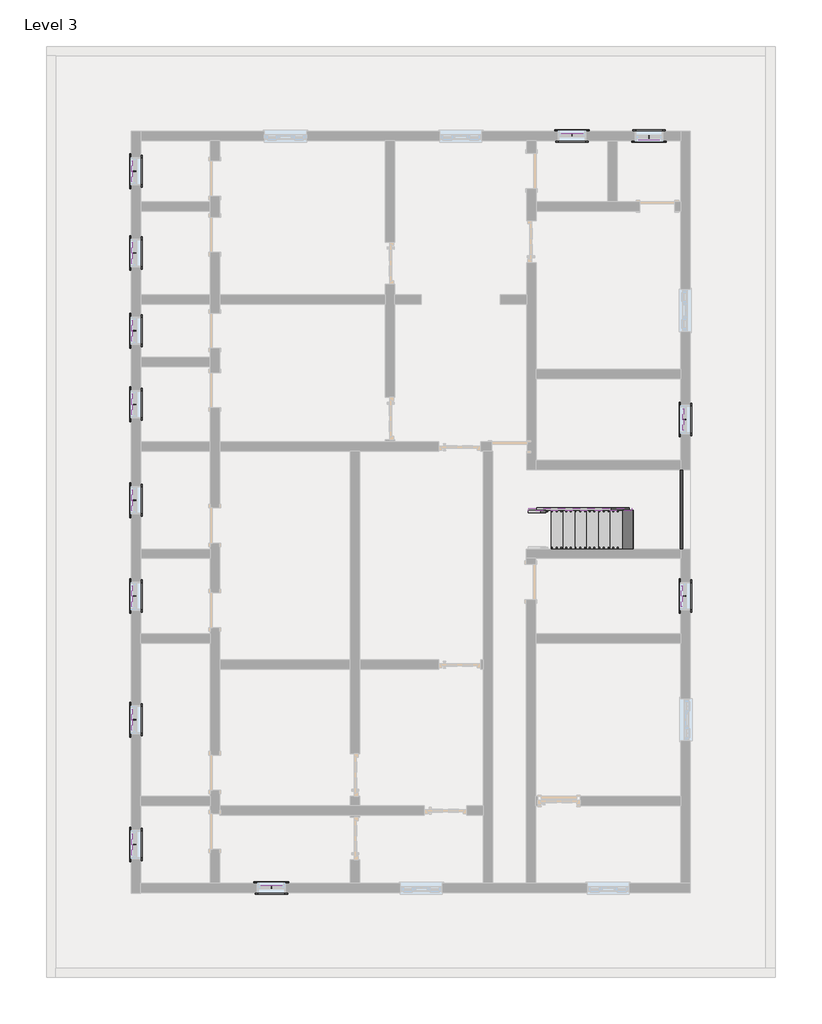
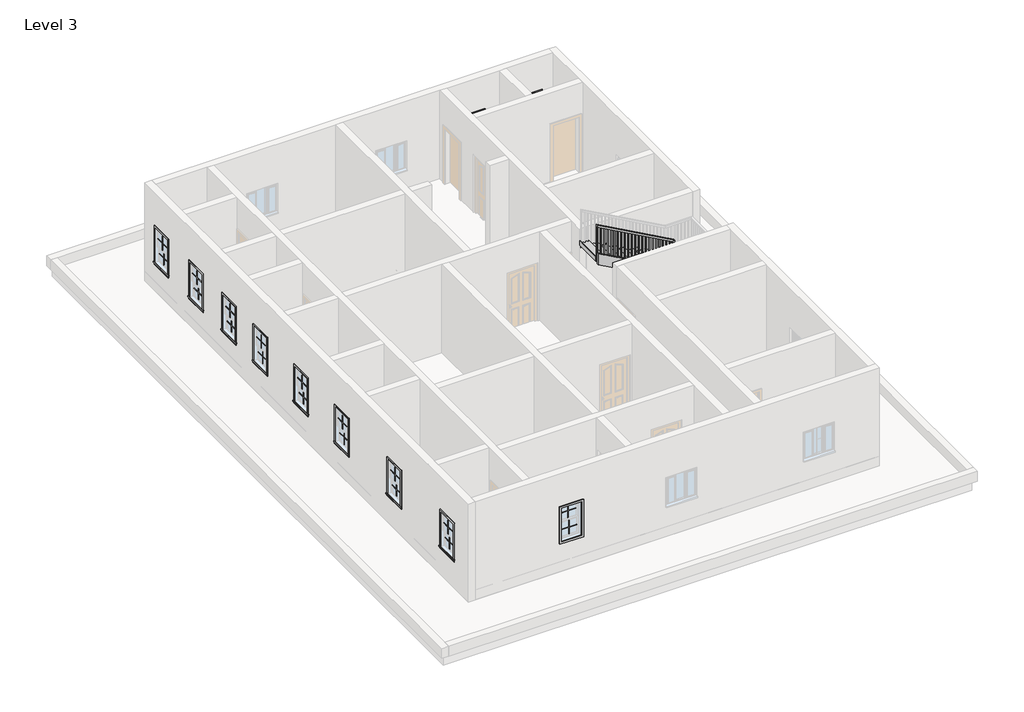
# One storey, part 3 of 3: 52 proxies, 5 members, 1 railing, 1 stair flight.
"""IFC4 building model written with IfcOpenShell, lengths in millimetres."""

from ifc_helpers import new_model, si_unit, frame, origin, place, context, project, spatial, polyline, outline, extrude, faceted_brep, transform, mapped, element, save
from components import muntin_pattern_2x2_muntin_pattern_2x2_eba6c5fb, trim_window_exterior_flat_with_sill_278e6a94, trim_window_interior_flat_picture_frame_e9fd5f45, stair_flight_fbd0abf4

model = new_model("IFC4")

# Units and contexts
model_context = context("Model", 3, world=origin())
ifc_project = project(units=[si_unit("LENGTHUNIT", "METRE", prefix="MILLI")], contexts=[model_context])

# Site, building, storey
site = spatial("IfcSite", under=ifc_project)
building = spatial("IfcBuilding", under=site)
storey = spatial("IfcBuildingStorey", under=building, Name="Level 3", Elevation=6096.0)

# Proxies
placement = place(None, origin())
muntin_pattern_2x2_muntin_pattern_2x2_shape = muntin_pattern_2x2_muntin_pattern_2x2_eba6c5fb(model_context)
element("IfcBuildingElementProxy", 1, Name="Muntin Pattern_2x2 : Muntin Pattern_2x2", ObjectType="Muntin Pattern_2x2 : Muntin Pattern_2x2", at=placement, inside=storey, context=model_context, shape_type="MappedRepresentation", body=[
    mapped(muntin_pattern_2x2_muntin_pattern_2x2_shape, transform((-10440.7626145, 6547.3404944, 7566.025), x_axis=(0.0, 1.0, 0.0), y_axis=(-1.0, 0.0, 0.0), z_axis=(0.0, 0.0, 1.0))),
])
element("IfcBuildingElementProxy", 2, Name="Muntin Pattern_2x2 : Muntin Pattern_2x2", ObjectType="Muntin Pattern_2x2 : Muntin Pattern_2x2", at=placement, inside=storey, context=model_context, shape_type="MappedRepresentation", body=[
    mapped(muntin_pattern_2x2_muntin_pattern_2x2_shape, transform((-10396.3126145, 6547.3404944, 7086.6), x_axis=(0.0, 1.0, 0.0), y_axis=(-1.0, 0.0, 0.0), z_axis=(0.0, 0.0, 1.0))),
])
element("IfcBuildingElementProxy", 3, Name="Muntin Pattern_2x2 : Muntin Pattern_2x2", ObjectType="Muntin Pattern_2x2 : Muntin Pattern_2x2", at=placement, inside=storey, context=model_context, shape_type="MappedRepresentation", body=[
    mapped(muntin_pattern_2x2_muntin_pattern_2x2_shape, transform((-10440.7626145, 4782.0404944, 7566.025), x_axis=(0.0, 1.0, 0.0), y_axis=(-1.0, 0.0, 0.0), z_axis=(0.0, 0.0, 1.0))),
])
element("IfcBuildingElementProxy", 4, Name="Muntin Pattern_2x2 : Muntin Pattern_2x2", ObjectType="Muntin Pattern_2x2 : Muntin Pattern_2x2", at=placement, inside=storey, context=model_context, shape_type="MappedRepresentation", body=[
    mapped(muntin_pattern_2x2_muntin_pattern_2x2_shape, transform((-10396.3126145, 4782.0404944, 7086.6), x_axis=(0.0, 1.0, 0.0), y_axis=(-1.0, 0.0, 0.0), z_axis=(0.0, 0.0, 1.0))),
])
element("IfcBuildingElementProxy", 5, Name="Muntin Pattern_2x2 : Muntin Pattern_2x2", ObjectType="Muntin Pattern_2x2 : Muntin Pattern_2x2", at=placement, inside=storey, context=model_context, shape_type="MappedRepresentation", body=[
    mapped(muntin_pattern_2x2_muntin_pattern_2x2_shape, transform((-10440.7626145, 3105.6404944, 7566.025), x_axis=(0.0, 1.0, 0.0), y_axis=(-1.0, 0.0, 0.0), z_axis=(0.0, 0.0, 1.0))),
])
element("IfcBuildingElementProxy", 6, Name="Muntin Pattern_2x2 : Muntin Pattern_2x2", ObjectType="Muntin Pattern_2x2 : Muntin Pattern_2x2", at=placement, inside=storey, context=model_context, shape_type="MappedRepresentation", body=[
    mapped(muntin_pattern_2x2_muntin_pattern_2x2_shape, transform((-10396.3126145, 3105.6404944, 7086.6), x_axis=(0.0, 1.0, 0.0), y_axis=(-1.0, 0.0, 0.0), z_axis=(0.0, 0.0, 1.0))),
])
element("IfcBuildingElementProxy", 7, Name="Muntin Pattern_2x2 : Muntin Pattern_2x2", ObjectType="Muntin Pattern_2x2 : Muntin Pattern_2x2", at=placement, inside=storey, context=model_context, shape_type="MappedRepresentation", body=[
    mapped(muntin_pattern_2x2_muntin_pattern_2x2_shape, transform((-10440.7626145, 1518.1404944, 7566.025), x_axis=(0.0, 1.0, 0.0), y_axis=(-1.0, 0.0, 0.0), z_axis=(0.0, 0.0, 1.0))),
])
element("IfcBuildingElementProxy", 8, Name="Muntin Pattern_2x2 : Muntin Pattern_2x2", ObjectType="Muntin Pattern_2x2 : Muntin Pattern_2x2", at=placement, inside=storey, context=model_context, shape_type="MappedRepresentation", body=[
    mapped(muntin_pattern_2x2_muntin_pattern_2x2_shape, transform((-10396.3126145, 1518.1404944, 7086.6), x_axis=(0.0, 1.0, 0.0), y_axis=(-1.0, 0.0, 0.0), z_axis=(0.0, 0.0, 1.0))),
])
element("IfcBuildingElementProxy", 9, Name="Muntin Pattern_2x2 : Muntin Pattern_2x2", ObjectType="Muntin Pattern_2x2 : Muntin Pattern_2x2", at=placement, inside=storey, context=model_context, shape_type="MappedRepresentation", body=[
    mapped(muntin_pattern_2x2_muntin_pattern_2x2_shape, transform((-10440.7626145, -551.9595056, 7566.025), x_axis=(0.0, 1.0, 0.0), y_axis=(-1.0, 0.0, 0.0), z_axis=(0.0, 0.0, 1.0))),
])
element("IfcBuildingElementProxy", 10, Name="Muntin Pattern_2x2 : Muntin Pattern_2x2", ObjectType="Muntin Pattern_2x2 : Muntin Pattern_2x2", at=placement, inside=storey, context=model_context, shape_type="MappedRepresentation", body=[
    mapped(muntin_pattern_2x2_muntin_pattern_2x2_shape, transform((-10396.3126145, -551.9595056, 7086.6), x_axis=(0.0, 1.0, 0.0), y_axis=(-1.0, 0.0, 0.0), z_axis=(0.0, 0.0, 1.0))),
])
element("IfcBuildingElementProxy", 11, Name="Muntin Pattern_2x2 : Muntin Pattern_2x2", ObjectType="Muntin Pattern_2x2 : Muntin Pattern_2x2", at=placement, inside=storey, context=model_context, shape_type="MappedRepresentation", body=[
    mapped(muntin_pattern_2x2_muntin_pattern_2x2_shape, transform((-10440.7626145, -2622.0595056, 7566.025), x_axis=(0.0, 1.0, 0.0), y_axis=(-1.0, 0.0, 0.0), z_axis=(0.0, 0.0, 1.0))),
])
element("IfcBuildingElementProxy", 12, Name="Muntin Pattern_2x2 : Muntin Pattern_2x2", ObjectType="Muntin Pattern_2x2 : Muntin Pattern_2x2", at=placement, inside=storey, context=model_context, shape_type="MappedRepresentation", body=[
    mapped(muntin_pattern_2x2_muntin_pattern_2x2_shape, transform((-10396.3126145, -2622.0595056, 7086.6), x_axis=(0.0, 1.0, 0.0), y_axis=(-1.0, 0.0, 0.0), z_axis=(0.0, 0.0, 1.0))),
])
element("IfcBuildingElementProxy", 13, Name="Muntin Pattern_2x2 : Muntin Pattern_2x2", ObjectType="Muntin Pattern_2x2 : Muntin Pattern_2x2", at=placement, inside=storey, context=model_context, shape_type="MappedRepresentation", body=[
    mapped(muntin_pattern_2x2_muntin_pattern_2x2_shape, transform((-10440.7626145, -5289.0595056, 7566.025), x_axis=(0.0, 1.0, 0.0), y_axis=(-1.0, 0.0, 0.0), z_axis=(0.0, 0.0, 1.0))),
])
element("IfcBuildingElementProxy", 14, Name="Muntin Pattern_2x2 : Muntin Pattern_2x2", ObjectType="Muntin Pattern_2x2 : Muntin Pattern_2x2", at=placement, inside=storey, context=model_context, shape_type="MappedRepresentation", body=[
    mapped(muntin_pattern_2x2_muntin_pattern_2x2_shape, transform((-10396.3126145, -5289.0595056, 7086.6), x_axis=(0.0, 1.0, 0.0), y_axis=(-1.0, 0.0, 0.0), z_axis=(0.0, 0.0, 1.0))),
])
element("IfcBuildingElementProxy", 15, Name="Muntin Pattern_2x2 : Muntin Pattern_2x2", ObjectType="Muntin Pattern_2x2 : Muntin Pattern_2x2", at=placement, inside=storey, context=model_context, shape_type="MappedRepresentation", body=[
    mapped(muntin_pattern_2x2_muntin_pattern_2x2_shape, transform((-10440.7626145, -7981.4595056, 7566.025), x_axis=(0.0, 1.0, 0.0), y_axis=(-1.0, 0.0, 0.0), z_axis=(0.0, 0.0, 1.0))),
])
element("IfcBuildingElementProxy", 16, Name="Muntin Pattern_2x2 : Muntin Pattern_2x2", ObjectType="Muntin Pattern_2x2 : Muntin Pattern_2x2", at=placement, inside=storey, context=model_context, shape_type="MappedRepresentation", body=[
    mapped(muntin_pattern_2x2_muntin_pattern_2x2_shape, transform((-10396.3126145, -7981.4595056, 7086.6), x_axis=(0.0, 1.0, 0.0), y_axis=(-1.0, 0.0, 0.0), z_axis=(0.0, 0.0, 1.0))),
])
element("IfcBuildingElementProxy", 17, Name="Muntin Pattern_2x2 : Muntin Pattern_2x2", ObjectType="Muntin Pattern_2x2 : Muntin Pattern_2x2", at=placement, inside=storey, context=model_context, shape_type="MappedRepresentation", body=[
    mapped(muntin_pattern_2x2_muntin_pattern_2x2_shape, transform((-7453.0876145, -8854.5845056, 7566.025), x_axis=(1.0, 0.0, 0.0), y_axis=(0.0, 1.0, 0.0), z_axis=(0.0, 0.0, 1.0))),
])
element("IfcBuildingElementProxy", 18, Name="Muntin Pattern_2x2 : Muntin Pattern_2x2", ObjectType="Muntin Pattern_2x2 : Muntin Pattern_2x2", at=placement, inside=storey, context=model_context, shape_type="MappedRepresentation", body=[
    mapped(muntin_pattern_2x2_muntin_pattern_2x2_shape, transform((-7453.0876145, -8899.0345056, 7086.6), x_axis=(1.0, 0.0, 0.0), y_axis=(0.0, 1.0, 0.0), z_axis=(0.0, 0.0, 1.0))),
])
element("IfcBuildingElementProxy", 19, Name="Muntin Pattern_2x2 : Muntin Pattern_2x2", ObjectType="Muntin Pattern_2x2 : Muntin Pattern_2x2", at=placement, inside=storey, context=model_context, shape_type="MappedRepresentation", body=[
    mapped(muntin_pattern_2x2_muntin_pattern_2x2_shape, transform((1421.0373855, -2622.0595056, 7566.025), x_axis=(0.0, 1.0, 0.0), y_axis=(-1.0, 0.0, 0.0), z_axis=(0.0, 0.0, 1.0))),
])
element("IfcBuildingElementProxy", 20, Name="Muntin Pattern_2x2 : Muntin Pattern_2x2", ObjectType="Muntin Pattern_2x2 : Muntin Pattern_2x2", at=placement, inside=storey, context=model_context, shape_type="MappedRepresentation", body=[
    mapped(muntin_pattern_2x2_muntin_pattern_2x2_shape, transform((1465.4873855, -2622.0595056, 7086.6), x_axis=(0.0, 1.0, 0.0), y_axis=(-1.0, 0.0, 0.0), z_axis=(0.0, 0.0, 1.0))),
])
element("IfcBuildingElementProxy", 21, Name="Muntin Pattern_2x2 : Muntin Pattern_2x2", ObjectType="Muntin Pattern_2x2 : Muntin Pattern_2x2", at=placement, inside=storey, context=model_context, shape_type="MappedRepresentation", body=[
    mapped(muntin_pattern_2x2_muntin_pattern_2x2_shape, transform((1421.0373855, 1190.4645364, 7566.025), x_axis=(0.0, 1.0, 0.0), y_axis=(-1.0, 0.0, 0.0), z_axis=(0.0, 0.0, 1.0))),
])
element("IfcBuildingElementProxy", 22, Name="Muntin Pattern_2x2 : Muntin Pattern_2x2", ObjectType="Muntin Pattern_2x2 : Muntin Pattern_2x2", at=placement, inside=storey, context=model_context, shape_type="MappedRepresentation", body=[
    mapped(muntin_pattern_2x2_muntin_pattern_2x2_shape, transform((1465.4873855, 1190.4645364, 7086.6), x_axis=(0.0, 1.0, 0.0), y_axis=(-1.0, 0.0, 0.0), z_axis=(0.0, 0.0, 1.0))),
])
element("IfcBuildingElementProxy", 23, Name="Muntin Pattern_2x2 : Muntin Pattern_2x2", ObjectType="Muntin Pattern_2x2 : Muntin Pattern_2x2", at=placement, inside=storey, context=model_context, shape_type="MappedRepresentation", body=[
    mapped(muntin_pattern_2x2_muntin_pattern_2x2_shape, transform((700.3123855, 7242.6654944, 7566.025), x_axis=(-1.0, 0.0, 0.0), y_axis=(0.0, -1.0, 0.0), z_axis=(0.0, 0.0, 1.0))),
])
element("IfcBuildingElementProxy", 24, Name="Muntin Pattern_2x2 : Muntin Pattern_2x2", ObjectType="Muntin Pattern_2x2 : Muntin Pattern_2x2", at=placement, inside=storey, context=model_context, shape_type="MappedRepresentation", body=[
    mapped(muntin_pattern_2x2_muntin_pattern_2x2_shape, transform((700.3123855, 7287.1154944, 7086.6), x_axis=(-1.0, 0.0, 0.0), y_axis=(0.0, -1.0, 0.0), z_axis=(0.0, 0.0, 1.0))),
])
element("IfcBuildingElementProxy", 25, Name="Muntin Pattern_2x2 : Muntin Pattern_2x2", ObjectType="Muntin Pattern_2x2 : Muntin Pattern_2x2", at=placement, inside=storey, context=model_context, shape_type="MappedRepresentation", body=[
    mapped(muntin_pattern_2x2_muntin_pattern_2x2_shape, transform((-963.3876145, 7376.0154944, 7566.025), x_axis=(1.0, 0.0, 0.0), y_axis=(0.0, 1.0, 0.0), z_axis=(0.0, 0.0, 1.0))),
])
element("IfcBuildingElementProxy", 26, Name="Muntin Pattern_2x2 : Muntin Pattern_2x2", ObjectType="Muntin Pattern_2x2 : Muntin Pattern_2x2", at=placement, inside=storey, context=model_context, shape_type="MappedRepresentation", body=[
    mapped(muntin_pattern_2x2_muntin_pattern_2x2_shape, transform((-963.3876145, 7331.5654944, 7086.6), x_axis=(1.0, 0.0, 0.0), y_axis=(0.0, 1.0, 0.0), z_axis=(0.0, 0.0, 1.0))),
])
trim_window_exterior_flat_with_sill_shape = trim_window_exterior_flat_with_sill_278e6a94(model_context)
element("IfcBuildingElementProxy", 27, Name="Trim-Window-Exterior-Flat : with Sill", ObjectType="Trim-Window-Exterior-Flat : with Sill", at=placement, inside=storey, context=model_context, shape_type="MappedRepresentation", body=[
    mapped(trim_window_exterior_flat_with_sill_shape, transform((-10475.6876145, 6547.3404944, 8077.2), x_axis=(0.0, -1.0, 0.0), y_axis=(0.0, 0.0, 1.0), z_axis=(-1.0, 0.0, 0.0))),
])
element("IfcBuildingElementProxy", 28, Name="Trim-Window-Exterior-Flat : with Sill", ObjectType="Trim-Window-Exterior-Flat : with Sill", at=placement, inside=storey, context=model_context, shape_type="MappedRepresentation", body=[
    mapped(trim_window_exterior_flat_with_sill_shape, transform((-10475.6876145, 4782.0404944, 8077.2), x_axis=(0.0, -1.0, 0.0), y_axis=(0.0, 0.0, 1.0), z_axis=(-1.0, 0.0, 0.0))),
])
element("IfcBuildingElementProxy", 29, Name="Trim-Window-Exterior-Flat : with Sill", ObjectType="Trim-Window-Exterior-Flat : with Sill", at=placement, inside=storey, context=model_context, shape_type="MappedRepresentation", body=[
    mapped(trim_window_exterior_flat_with_sill_shape, transform((-10475.6876145, 3105.6404944, 8077.2), x_axis=(0.0, -1.0, 0.0), y_axis=(0.0, 0.0, 1.0), z_axis=(-1.0, 0.0, 0.0))),
])
element("IfcBuildingElementProxy", 30, Name="Trim-Window-Exterior-Flat : with Sill", ObjectType="Trim-Window-Exterior-Flat : with Sill", at=placement, inside=storey, context=model_context, shape_type="MappedRepresentation", body=[
    mapped(trim_window_exterior_flat_with_sill_shape, transform((-10475.6876145, 1518.1404944, 8077.2), x_axis=(0.0, -1.0, 0.0), y_axis=(0.0, 0.0, 1.0), z_axis=(-1.0, 0.0, 0.0))),
])
element("IfcBuildingElementProxy", 31, Name="Trim-Window-Exterior-Flat : with Sill", ObjectType="Trim-Window-Exterior-Flat : with Sill", at=placement, inside=storey, context=model_context, shape_type="MappedRepresentation", body=[
    mapped(trim_window_exterior_flat_with_sill_shape, transform((-10475.6876145, -551.9595056, 8077.2), x_axis=(0.0, -1.0, 0.0), y_axis=(0.0, 0.0, 1.0), z_axis=(-1.0, 0.0, 0.0))),
])
element("IfcBuildingElementProxy", 32, Name="Trim-Window-Exterior-Flat : with Sill", ObjectType="Trim-Window-Exterior-Flat : with Sill", at=placement, inside=storey, context=model_context, shape_type="MappedRepresentation", body=[
    mapped(trim_window_exterior_flat_with_sill_shape, transform((-10475.6876145, -2622.0595056, 8077.2), x_axis=(0.0, -1.0, 0.0), y_axis=(0.0, 0.0, 1.0), z_axis=(-1.0, 0.0, 0.0))),
])
element("IfcBuildingElementProxy", 33, Name="Trim-Window-Exterior-Flat : with Sill", ObjectType="Trim-Window-Exterior-Flat : with Sill", at=placement, inside=storey, context=model_context, shape_type="MappedRepresentation", body=[
    mapped(trim_window_exterior_flat_with_sill_shape, transform((-10475.6876145, -5289.0595056, 8077.2), x_axis=(0.0, -1.0, 0.0), y_axis=(0.0, 0.0, 1.0), z_axis=(-1.0, 0.0, 0.0))),
])
element("IfcBuildingElementProxy", 34, Name="Trim-Window-Exterior-Flat : with Sill", ObjectType="Trim-Window-Exterior-Flat : with Sill", at=placement, inside=storey, context=model_context, shape_type="MappedRepresentation", body=[
    mapped(trim_window_exterior_flat_with_sill_shape, transform((-10475.6876145, -7981.4595056, 8077.2), x_axis=(0.0, -1.0, 0.0), y_axis=(0.0, 0.0, 1.0), z_axis=(-1.0, 0.0, 0.0))),
])
element("IfcBuildingElementProxy", 35, Name="Trim-Window-Exterior-Flat : with Sill", ObjectType="Trim-Window-Exterior-Flat : with Sill", at=placement, inside=storey, context=model_context, shape_type="MappedRepresentation", body=[
    mapped(trim_window_exterior_flat_with_sill_shape, transform((-7453.0876145, -8819.6595056, 8077.2), x_axis=(-1.0, 0.0, 0.0), y_axis=(0.0, 0.0, 1.0), z_axis=(0.0, 1.0, 0.0))),
])
element("IfcBuildingElementProxy", 36, Name="Trim-Window-Exterior-Flat : with Sill", ObjectType="Trim-Window-Exterior-Flat : with Sill", at=placement, inside=storey, context=model_context, shape_type="MappedRepresentation", body=[
    mapped(trim_window_exterior_flat_with_sill_shape, transform((1386.1123855, -2622.0595056, 8077.2), x_axis=(0.0, -1.0, 0.0), y_axis=(0.0, 0.0, 1.0), z_axis=(-1.0, 0.0, 0.0))),
])
element("IfcBuildingElementProxy", 37, Name="Trim-Window-Exterior-Flat : with Sill", ObjectType="Trim-Window-Exterior-Flat : with Sill", at=placement, inside=storey, context=model_context, shape_type="MappedRepresentation", body=[
    mapped(trim_window_exterior_flat_with_sill_shape, transform((1386.1123855, 1190.4645364, 8077.2), x_axis=(0.0, -1.0, 0.0), y_axis=(0.0, 0.0, 1.0), z_axis=(-1.0, 0.0, 0.0))),
])
element("IfcBuildingElementProxy", 38, Name="Trim-Window-Exterior-Flat : with Sill", ObjectType="Trim-Window-Exterior-Flat : with Sill", at=placement, inside=storey, context=model_context, shape_type="MappedRepresentation", body=[
    mapped(trim_window_exterior_flat_with_sill_shape, transform((700.3123855, 7207.7404944, 8077.2), x_axis=(1.0, 0.0, 0.0), y_axis=(0.0, 0.0, 1.0), z_axis=(0.0, -1.0, 0.0))),
])
element("IfcBuildingElementProxy", 39, Name="Trim-Window-Exterior-Flat : with Sill", ObjectType="Trim-Window-Exterior-Flat : with Sill", at=placement, inside=storey, context=model_context, shape_type="MappedRepresentation", body=[
    mapped(trim_window_exterior_flat_with_sill_shape, transform((-963.3876145, 7410.9404944, 8077.2), x_axis=(-1.0, 0.0, 0.0), y_axis=(0.0, 0.0, 1.0), z_axis=(0.0, 1.0, 0.0))),
])
trim_window_interior_flat_picture_frame_shape = trim_window_interior_flat_picture_frame_e9fd5f45(model_context)
element("IfcBuildingElementProxy", 40, Name="Trim-Window-Interior-Flat : Picture Frame", ObjectType="Trim-Window-Interior-Flat : Picture Frame", at=placement, inside=storey, context=model_context, shape_type="MappedRepresentation", body=[
    mapped(trim_window_interior_flat_picture_frame_shape, transform((-10272.4876145, 6547.3404944, 8077.2), x_axis=(0.0, 1.0, 0.0), y_axis=(0.0, 0.0, 1.0), z_axis=(1.0, 0.0, 0.0))),
])
element("IfcBuildingElementProxy", 41, Name="Trim-Window-Interior-Flat : Picture Frame", ObjectType="Trim-Window-Interior-Flat : Picture Frame", at=placement, inside=storey, context=model_context, shape_type="MappedRepresentation", body=[
    mapped(trim_window_interior_flat_picture_frame_shape, transform((-10272.4876145, 4782.0404944, 8077.2), x_axis=(0.0, 1.0, 0.0), y_axis=(0.0, 0.0, 1.0), z_axis=(1.0, 0.0, 0.0))),
])
element("IfcBuildingElementProxy", 42, Name="Trim-Window-Interior-Flat : Picture Frame", ObjectType="Trim-Window-Interior-Flat : Picture Frame", at=placement, inside=storey, context=model_context, shape_type="MappedRepresentation", body=[
    mapped(trim_window_interior_flat_picture_frame_shape, transform((-10272.4876145, 3105.6404944, 8077.2), x_axis=(0.0, 1.0, 0.0), y_axis=(0.0, 0.0, 1.0), z_axis=(1.0, 0.0, 0.0))),
])
element("IfcBuildingElementProxy", 43, Name="Trim-Window-Interior-Flat : Picture Frame", ObjectType="Trim-Window-Interior-Flat : Picture Frame", at=placement, inside=storey, context=model_context, shape_type="MappedRepresentation", body=[
    mapped(trim_window_interior_flat_picture_frame_shape, transform((-10272.4876145, 1518.1404944, 8077.2), x_axis=(0.0, 1.0, 0.0), y_axis=(0.0, 0.0, 1.0), z_axis=(1.0, 0.0, 0.0))),
])
element("IfcBuildingElementProxy", 44, Name="Trim-Window-Interior-Flat : Picture Frame", ObjectType="Trim-Window-Interior-Flat : Picture Frame", at=placement, inside=storey, context=model_context, shape_type="MappedRepresentation", body=[
    mapped(trim_window_interior_flat_picture_frame_shape, transform((-10272.4876145, -551.9595056, 8077.2), x_axis=(0.0, 1.0, 0.0), y_axis=(0.0, 0.0, 1.0), z_axis=(1.0, 0.0, 0.0))),
])
element("IfcBuildingElementProxy", 45, Name="Trim-Window-Interior-Flat : Picture Frame", ObjectType="Trim-Window-Interior-Flat : Picture Frame", at=placement, inside=storey, context=model_context, shape_type="MappedRepresentation", body=[
    mapped(trim_window_interior_flat_picture_frame_shape, transform((-10272.4876145, -2622.0595056, 8077.2), x_axis=(0.0, 1.0, 0.0), y_axis=(0.0, 0.0, 1.0), z_axis=(1.0, 0.0, 0.0))),
])
element("IfcBuildingElementProxy", 46, Name="Trim-Window-Interior-Flat : Picture Frame", ObjectType="Trim-Window-Interior-Flat : Picture Frame", at=placement, inside=storey, context=model_context, shape_type="MappedRepresentation", body=[
    mapped(trim_window_interior_flat_picture_frame_shape, transform((-10272.4876145, -5289.0595056, 8077.2), x_axis=(0.0, 1.0, 0.0), y_axis=(0.0, 0.0, 1.0), z_axis=(1.0, 0.0, 0.0))),
])
element("IfcBuildingElementProxy", 47, Name="Trim-Window-Interior-Flat : Picture Frame", ObjectType="Trim-Window-Interior-Flat : Picture Frame", at=placement, inside=storey, context=model_context, shape_type="MappedRepresentation", body=[
    mapped(trim_window_interior_flat_picture_frame_shape, transform((-10272.4876145, -7981.4595056, 8077.2), x_axis=(0.0, 1.0, 0.0), y_axis=(0.0, 0.0, 1.0), z_axis=(1.0, 0.0, 0.0))),
])
element("IfcBuildingElementProxy", 48, Name="Trim-Window-Interior-Flat : Picture Frame", ObjectType="Trim-Window-Interior-Flat : Picture Frame", at=placement, inside=storey, context=model_context, shape_type="MappedRepresentation", body=[
    mapped(trim_window_interior_flat_picture_frame_shape, transform((-7453.0876145, -9022.8595056, 8077.2), x_axis=(1.0, 0.0, 0.0), y_axis=(0.0, 0.0, 1.0), z_axis=(0.0, -1.0, 0.0))),
])
element("IfcBuildingElementProxy", 49, Name="Trim-Window-Interior-Flat : Picture Frame", ObjectType="Trim-Window-Interior-Flat : Picture Frame", at=placement, inside=storey, context=model_context, shape_type="MappedRepresentation", body=[
    mapped(trim_window_interior_flat_picture_frame_shape, transform((1589.3123855, -2622.0595056, 8077.2), x_axis=(0.0, 1.0, 0.0), y_axis=(0.0, 0.0, 1.0), z_axis=(1.0, 0.0, 0.0))),
])
element("IfcBuildingElementProxy", 50, Name="Trim-Window-Interior-Flat : Picture Frame", ObjectType="Trim-Window-Interior-Flat : Picture Frame", at=placement, inside=storey, context=model_context, shape_type="MappedRepresentation", body=[
    mapped(trim_window_interior_flat_picture_frame_shape, transform((1589.3123855, 1190.4645364, 8077.2), x_axis=(0.0, 1.0, 0.0), y_axis=(0.0, 0.0, 1.0), z_axis=(1.0, 0.0, 0.0))),
])
element("IfcBuildingElementProxy", 51, Name="Trim-Window-Interior-Flat : Picture Frame", ObjectType="Trim-Window-Interior-Flat : Picture Frame", at=placement, inside=storey, context=model_context, shape_type="MappedRepresentation", body=[
    mapped(trim_window_interior_flat_picture_frame_shape, transform((700.3123855, 7410.9404944, 8077.2), x_axis=(-1.0, 0.0, 0.0), y_axis=(0.0, 0.0, 1.0), z_axis=(0.0, 1.0, 0.0))),
])
element("IfcBuildingElementProxy", 52, Name="Trim-Window-Interior-Flat : Picture Frame", ObjectType="Trim-Window-Interior-Flat : Picture Frame", at=placement, inside=storey, context=model_context, shape_type="MappedRepresentation", body=[
    mapped(trim_window_interior_flat_picture_frame_shape, transform((-963.3876145, 7207.7404944, 8077.2), x_axis=(1.0, 0.0, 0.0), y_axis=(0.0, 0.0, 1.0), z_axis=(0.0, -1.0, 0.0))),
])

# Members
element("IfcMember", 53, ObjectType="Stringer - 2\" Width", at=placement, inside=storey, context=model_context, shape_type="SweptSolid", body=[
    extrude(outline(polyline([(6306.6757607, -1903.1876145), (6096.0, -1903.1876145), (6096.0, -1654.2050647), (7161.4963497, 274.6830625), (7509.7073019, 274.6830625), (6306.6757607, -1903.1876145)])), frame((0.0, -767.8595056, 0.0), z_axis=(0.0, 1.0, 0.0), x_axis=(0.0, 0.0, 1.0)), (0.0, 0.0, 1.0), 50.8),
])
element("IfcMember", 54, ObjectType="Stringer - 2\" Width", at=placement, inside=storey, context=model_context, shape_type="SweptSolid", body=[
    extrude(outline(polyline([(7326.7177047, 325.4830625), (7674.928657, 325.4830625), (8906.0215532, -1903.1876145), (8557.8106009, -1903.1876145), (7326.7177047, 325.4830625)])), frame((0.0, -780.5595056, 0.0), z_axis=(0.0, 1.0, 0.0), x_axis=(0.0, 0.0, 1.0)), (0.0, 0.0, 1.0), 50.8),
])
element("IfcMember", 55, ObjectType="Stringer - 2\" Width", at=placement, inside=storey, context=model_context, shape_type="SweptSolid", body=[
    extrude(outline(polyline([(6306.6757607, -1903.1876145), (6096.0, -1903.1876145), (6096.0, -1654.2050647), (7543.8, 966.7745674), (7543.8, 336.4017165), (6306.6757607, -1903.1876145)])), frame((0.0, -1656.8595056, 0.0), z_axis=(0.0, 1.0, 0.0), x_axis=(0.0, 0.0, 1.0)), (0.0, 0.0, 1.0), 50.8),
])
element("IfcMember", 56, ObjectType="Stringer - 2\" Width", at=placement, inside=storey, context=model_context, shape_type="SweptSolid", body=[
    extrude(outline(polyline([(1424.2123855, -1656.8595056), (1373.4123855, -1656.8595056), (1373.4123855, 108.4404944), (1424.2123855, 108.4404944), (1424.2123855, -1656.8595056)])), frame((0.0, 0.0, 7239.0), z_axis=(0.0, 0.0, 1.0), x_axis=(1.0, 0.0, 0.0)), (0.0, 0.0, 1.0), 304.8),
])
element("IfcMember", 57, ObjectType="Stringer - 2\" Width", at=placement, inside=storey, context=model_context, shape_type="SweptSolid", body=[
    extrude(outline(polyline([(7239.0, 1114.6529278), (8906.0215532, -1903.1876145), (8557.8106009, -1903.1876145), (7239.0, 484.2800769), (7239.0, 1114.6529278)])), frame((0.0, 108.4404944, 0.0), z_axis=(0.0, 1.0, 0.0), x_axis=(0.0, 0.0, 1.0)), (0.0, 0.0, 1.0), 50.8),
])

# Railing
element("IfcRailing", 58, ObjectType="Handrail - Rectangular", at=placement, inside=storey, context=model_context, shape_type="SolidModel", body=[
    faceted_brep([(-1903.1876145, -767.8595056, 7147.56), (-1903.1876145, -767.8595056, 7089.4879132), (-1903.1876145, -818.6595056, 7089.4879132), (-1903.1876145, -818.6595056, 7147.56), (325.4830625, -767.8595056, 8382.0), (325.4830625, -818.6595056, 8382.0), (325.4830625, -818.6595056, 8323.9279132), (325.4830625, -767.8595056, 8323.9279132)], [[[0, 1, 2, 3]], [[4, 5, 6, 7]], [[1, 0, 4, 7]], [[2, 1, 7, 6]], [[3, 2, 6, 5]], [[0, 3, 5, 4]]]),
    faceted_brep([(325.4830625, -818.6595056, 8382.0), (325.4830625, -818.6595056, 8331.2), (376.2830625, -818.6595056, 8331.2), (376.2830625, -818.6595056, 8382.0), (325.4830625, -729.7595056, 8382.0), (376.2830625, -729.7595056, 8382.0), (376.2830625, -678.9595056, 8331.2), (325.4830625, -678.9595056, 8331.2)], [[[0, 1, 2, 3]], [[4, 5, 6, 7]], [[1, 0, 4, 7]], [[2, 1, 7, 6]], [[3, 2, 6, 5]], [[0, 3, 5, 4]]]),
    faceted_brep([(325.4830625, -729.7595056, 8382.0), (325.4830625, -678.9595056, 8331.2), (376.2830625, -678.9595056, 8331.2), (376.2830625, -729.7595056, 8382.0), (325.4830625, -729.7595056, 8461.0879132), (376.2830625, -729.7595056, 8491.0223516), (376.2830625, -678.9595056, 8491.0223516), (325.4830625, -678.9595056, 8461.0879132)], [[[0, 1, 2, 3]], [[4, 5, 6, 7]], [[1, 0, 4, 7]], [[2, 1, 7, 6]], [[3, 2, 6, 5]], [[0, 3, 5, 4]]]),
    faceted_brep([(376.2830625, -729.7595056, 8491.0223516), (325.4830625, -729.7595056, 8461.0879132), (325.4830625, -678.9595056, 8461.0879132), (376.2830625, -678.9595056, 8491.0223516), (-1903.1876145, -729.7595056, 9753.6), (-1903.1876145, -678.9595056, 9753.6), (-1903.1876145, -678.9595056, 9695.5279132), (-1903.1876145, -729.7595056, 9695.5279132)], [[[0, 1, 2, 3]], [[4, 5, 6, 7]], [[1, 0, 4, 7]], [[2, 1, 7, 6]], [[3, 2, 6, 5]], [[0, 3, 5, 4]]]),
    extrude(outline(polyline([(9690.3072849, -1893.8419375), (8702.04, -1893.8419375), (8702.04, -1874.7919375), (9679.7556667, -1874.7919375), (9690.3072849, -1893.8419375)])), frame((0.0, -713.8845056, 0.0), z_axis=(0.0, 1.0, 0.0), x_axis=(0.0, 0.0, 1.0)), (0.0, 0.0, 1.0), 19.05),
    extrude(outline(polyline([(9634.031988, -1792.2419375), (8702.04, -1792.2419375), (8702.04, -1773.1919375), (9623.4803699, -1773.1919375), (9634.031988, -1792.2419375)])), frame((0.0, -713.8845056, 0.0), z_axis=(0.0, 1.0, 0.0), x_axis=(0.0, 0.0, 1.0)), (0.0, 0.0, 1.0), 19.05),
    extrude(outline(polyline([(9577.7125465, -1690.6419375), (8702.04, -1690.6419375), (8702.04, -1671.5919375), (9567.1609284, -1671.5919375), (9577.7125465, -1690.6419375)])), frame((0.0, -713.8845056, 0.0), z_axis=(0.0, 1.0, 0.0), x_axis=(0.0, 0.0, 1.0)), (0.0, 0.0, 1.0), 19.05),
    extrude(outline(polyline([(9521.4813943, -1589.0419375), (8564.88, -1589.0419375), (8564.88, -1569.9919375), (9510.9297761, -1569.9919375), (9521.4813943, -1589.0419375)])), frame((0.0, -713.8845056, 0.0), z_axis=(0.0, 1.0, 0.0), x_axis=(0.0, 0.0, 1.0)), (0.0, 0.0, 1.0), 19.05),
    extrude(outline(polyline([(9465.2060974, -1487.4419375), (8564.88, -1487.4419375), (8564.88, -1468.3919375), (9454.6544792, -1468.3919375), (9465.2060974, -1487.4419375)])), frame((0.0, -713.8845056, 0.0), z_axis=(0.0, 1.0, 0.0), x_axis=(0.0, 0.0, 1.0)), (0.0, 0.0, 1.0), 19.05),
    extrude(outline(polyline([(9408.9308005, -1385.8419375), (8427.72, -1385.8419375), (8427.72, -1366.7919375), (9398.3791823, -1366.7919375), (9408.9308005, -1385.8419375)])), frame((0.0, -713.8845056, 0.0), z_axis=(0.0, 1.0, 0.0), x_axis=(0.0, 0.0, 1.0)), (0.0, 0.0, 1.0), 19.05),
    extrude(outline(polyline([(9352.6555036, -1284.2419375), (8427.72, -1284.2419375), (8427.72, -1265.1919375), (9342.1038855, -1265.1919375), (9352.6555036, -1284.2419375)])), frame((0.0, -713.8845056, 0.0), z_axis=(0.0, 1.0, 0.0), x_axis=(0.0, 0.0, 1.0)), (0.0, 0.0, 1.0), 19.05),
    extrude(outline(polyline([(9296.3802067, -1182.6419375), (8427.72, -1182.6419375), (8427.72, -1163.5919375), (9285.8285886, -1163.5919375), (9296.3802067, -1182.6419375)])), frame((0.0, -713.8845056, 0.0), z_axis=(0.0, 1.0, 0.0), x_axis=(0.0, 0.0, 1.0)), (0.0, 0.0, 1.0), 19.05),
    extrude(outline(polyline([(9240.1049099, -1081.0419375), (8290.56, -1081.0419375), (8290.56, -1061.9919375), (9229.5532917, -1061.9919375), (9240.1049099, -1081.0419375)])), frame((0.0, -713.8845056, 0.0), z_axis=(0.0, 1.0, 0.0), x_axis=(0.0, 0.0, 1.0)), (0.0, 0.0, 1.0), 19.05),
    extrude(outline(polyline([(9183.829613, -979.4419375), (8290.56, -979.4419375), (8290.56, -960.3919375), (9173.2779948, -960.3919375), (9183.829613, -979.4419375)])), frame((0.0, -713.8845056, 0.0), z_axis=(0.0, 1.0, 0.0), x_axis=(0.0, 0.0, 1.0)), (0.0, 0.0, 1.0), 19.05),
    extrude(outline(polyline([(9127.5543161, -877.8419375), (8153.4, -877.8419375), (8153.4, -858.7919375), (9117.0026979, -858.7919375), (9127.5543161, -877.8419375)])), frame((0.0, -713.8845056, 0.0), z_axis=(0.0, 1.0, 0.0), x_axis=(0.0, 0.0, 1.0)), (0.0, 0.0, 1.0), 19.05),
    extrude(outline(polyline([(9071.2790192, -776.2419375), (8153.4, -776.2419375), (8153.4, -757.1919375), (9060.727401, -757.1919375), (9071.2790192, -776.2419375)])), frame((0.0, -713.8845056, 0.0), z_axis=(0.0, 1.0, 0.0), x_axis=(0.0, 0.0, 1.0)), (0.0, 0.0, 1.0), 19.05),
    extrude(outline(polyline([(9015.0478669, -674.6419375), (8153.4, -674.6419375), (8153.4, -655.5919375), (9004.4962488, -655.5919375), (9015.0478669, -674.6419375)])), frame((0.0, -713.8845056, 0.0), z_axis=(0.0, 1.0, 0.0), x_axis=(0.0, 0.0, 1.0)), (0.0, 0.0, 1.0), 19.05),
    extrude(outline(polyline([(8958.77257, -573.0419375), (8016.24, -573.0419375), (8016.24, -553.9919375), (8948.2209519, -553.9919375), (8958.77257, -573.0419375)])), frame((0.0, -713.8845056, 0.0), z_axis=(0.0, 1.0, 0.0), x_axis=(0.0, 0.0, 1.0)), (0.0, 0.0, 1.0), 19.05),
    extrude(outline(polyline([(8902.4972732, -471.4419375), (8016.24, -471.4419375), (8016.24, -452.3919375), (8891.945655, -452.3919375), (8902.4972732, -471.4419375)])), frame((0.0, -713.8845056, 0.0), z_axis=(0.0, 1.0, 0.0), x_axis=(0.0, 0.0, 1.0)), (0.0, 0.0, 1.0), 19.05),
    extrude(outline(polyline([(8846.2219763, -369.8419375), (7879.08, -369.8419375), (7879.08, -350.7919375), (8835.6703581, -350.7919375), (8846.2219763, -369.8419375)])), frame((0.0, -713.8845056, 0.0), z_axis=(0.0, 1.0, 0.0), x_axis=(0.0, 0.0, 1.0)), (0.0, 0.0, 1.0), 19.05),
    extrude(outline(polyline([(8789.9466794, -268.2419375), (7879.08, -268.2419375), (7879.08, -249.1919375), (8779.3950612, -249.1919375), (8789.9466794, -268.2419375)])), frame((0.0, -713.8845056, 0.0), z_axis=(0.0, 1.0, 0.0), x_axis=(0.0, 0.0, 1.0)), (0.0, 0.0, 1.0), 19.05),
    extrude(outline(polyline([(8733.6713825, -166.6419375), (7879.08, -166.6419375), (7879.08, -147.5919375), (8723.1197643, -147.5919375), (8733.6713825, -166.6419375)])), frame((0.0, -713.8845056, 0.0), z_axis=(0.0, 1.0, 0.0), x_axis=(0.0, 0.0, 1.0)), (0.0, 0.0, 1.0), 19.05),
    extrude(outline(polyline([(8677.3960856, -65.0419375), (7741.92, -65.0419375), (7741.92, -45.9919375), (8666.8444675, -45.9919375), (8677.3960856, -65.0419375)])), frame((0.0, -713.8845056, 0.0), z_axis=(0.0, 1.0, 0.0), x_axis=(0.0, 0.0, 1.0)), (0.0, 0.0, 1.0), 19.05),
    extrude(outline(polyline([(8621.1207888, 36.5580625), (7741.92, 36.5580625), (7741.92, 55.6080625), (8610.5691706, 55.6080625), (8621.1207888, 36.5580625)])), frame((0.0, -713.8845056, 0.0), z_axis=(0.0, 1.0, 0.0), x_axis=(0.0, 0.0, 1.0)), (0.0, 0.0, 1.0), 19.05),
    extrude(outline(polyline([(8564.8454919, 138.1580625), (7604.76, 138.1580625), (7604.76, 157.2080625), (8554.2938737, 157.2080625), (8564.8454919, 138.1580625)])), frame((0.0, -713.8845056, 0.0), z_axis=(0.0, 1.0, 0.0), x_axis=(0.0, 0.0, 1.0)), (0.0, 0.0, 1.0), 19.05),
    extrude(outline(polyline([(8508.570195, 239.7580625), (7604.76, 239.7580625), (7604.76, 258.8080625), (8498.0185768, 258.8080625), (8508.570195, 239.7580625)])), frame((0.0, -713.8845056, 0.0), z_axis=(0.0, 1.0, 0.0), x_axis=(0.0, 0.0, 1.0)), (0.0, 0.0, 1.0), 19.05),
    extrude(outline(polyline([(8322.2686355, 322.4873855), (7467.6, 322.4873855), (7467.6, 341.5373855), (8332.8202537, 341.5373855), (8322.2686355, 322.4873855)])), frame((0.0, -802.7845056, 0.0), z_axis=(0.0, 1.0, 0.0), x_axis=(0.0, 0.0, 1.0)), (0.0, 0.0, 1.0), 19.05),
    extrude(outline(polyline([(8265.9933387, 220.8873855), (7330.44, 220.8873855), (7330.44, 239.9373855), (8276.5449568, 239.9373855), (8265.9933387, 220.8873855)])), frame((0.0, -802.7845056, 0.0), z_axis=(0.0, 1.0, 0.0), x_axis=(0.0, 0.0, 1.0)), (0.0, 0.0, 1.0), 19.05),
    extrude(outline(polyline([(8209.7180418, 119.2873855), (7330.44, 119.2873855), (7330.44, 138.3373855), (8220.2696599, 138.3373855), (8209.7180418, 119.2873855)])), frame((0.0, -802.7845056, 0.0), z_axis=(0.0, 1.0, 0.0), x_axis=(0.0, 0.0, 1.0)), (0.0, 0.0, 1.0), 19.05),
    extrude(outline(polyline([(8153.4427449, 17.6873855), (7193.28, 17.6873855), (7193.28, 36.7373855), (8163.9943631, 36.7373855), (8153.4427449, 17.6873855)])), frame((0.0, -802.7845056, 0.0), z_axis=(0.0, 1.0, 0.0), x_axis=(0.0, 0.0, 1.0)), (0.0, 0.0, 1.0), 19.05),
    extrude(outline(polyline([(8097.167448, -83.9126145), (7193.28, -83.9126145), (7193.28, -64.8626145), (8107.7190662, -64.8626145), (8097.167448, -83.9126145)])), frame((0.0, -802.7845056, 0.0), z_axis=(0.0, 1.0, 0.0), x_axis=(0.0, 0.0, 1.0)), (0.0, 0.0, 1.0), 19.05),
    extrude(outline(polyline([(8040.8921511, -185.5126145), (7056.12, -185.5126145), (7056.12, -166.4626145), (8051.4437693, -166.4626145), (8040.8921511, -185.5126145)])), frame((0.0, -802.7845056, 0.0), z_axis=(0.0, 1.0, 0.0), x_axis=(0.0, 0.0, 1.0)), (0.0, 0.0, 1.0), 19.05),
    extrude(outline(polyline([(7984.6168543, -287.1126145), (7056.12, -287.1126145), (7056.12, -268.0626145), (7995.1684724, -268.0626145), (7984.6168543, -287.1126145)])), frame((0.0, -802.7845056, 0.0), z_axis=(0.0, 1.0, 0.0), x_axis=(0.0, 0.0, 1.0)), (0.0, 0.0, 1.0), 19.05),
    extrude(outline(polyline([(7928.3415574, -388.7126145), (7056.12, -388.7126145), (7056.12, -369.6626145), (7938.8931755, -369.6626145), (7928.3415574, -388.7126145)])), frame((0.0, -802.7845056, 0.0), z_axis=(0.0, 1.0, 0.0), x_axis=(0.0, 0.0, 1.0)), (0.0, 0.0, 1.0), 19.05),
    extrude(outline(polyline([(7872.0662605, -490.3126145), (6918.96, -490.3126145), (6918.96, -471.2626145), (7882.6178787, -471.2626145), (7872.0662605, -490.3126145)])), frame((0.0, -802.7845056, 0.0), z_axis=(0.0, 1.0, 0.0), x_axis=(0.0, 0.0, 1.0)), (0.0, 0.0, 1.0), 19.05),
    extrude(outline(polyline([(7815.7909636, -591.9126145), (6918.96, -591.9126145), (6918.96, -572.8626145), (7826.3425818, -572.8626145), (7815.7909636, -591.9126145)])), frame((0.0, -802.7845056, 0.0), z_axis=(0.0, 1.0, 0.0), x_axis=(0.0, 0.0, 1.0)), (0.0, 0.0, 1.0), 19.05),
    extrude(outline(polyline([(7759.5156667, -693.5126145), (6781.8, -693.5126145), (6781.8, -674.4626145), (7770.0672849, -674.4626145), (7759.5156667, -693.5126145)])), frame((0.0, -802.7845056, 0.0), z_axis=(0.0, 1.0, 0.0), x_axis=(0.0, 0.0, 1.0)), (0.0, 0.0, 1.0), 19.05),
    extrude(outline(polyline([(7703.2403699, -795.1126145), (6781.8, -795.1126145), (6781.8, -776.0626145), (7713.791988, -776.0626145), (7703.2403699, -795.1126145)])), frame((0.0, -802.7845056, 0.0), z_axis=(0.0, 1.0, 0.0), x_axis=(0.0, 0.0, 1.0)), (0.0, 0.0, 1.0), 19.05),
    extrude(outline(polyline([(7646.9209284, -896.7126145), (6781.8, -896.7126145), (6781.8, -877.6626145), (7657.4725466, -877.6626145), (7646.9209284, -896.7126145)])), frame((0.0, -802.7845056, 0.0), z_axis=(0.0, 1.0, 0.0), x_axis=(0.0, 0.0, 1.0)), (0.0, 0.0, 1.0), 19.05),
    extrude(outline(polyline([(7590.6897761, -998.3126145), (6644.64, -998.3126145), (6644.64, -979.2626145), (7601.2413943, -979.2626145), (7590.6897761, -998.3126145)])), frame((0.0, -802.7845056, 0.0), z_axis=(0.0, 1.0, 0.0), x_axis=(0.0, 0.0, 1.0)), (0.0, 0.0, 1.0), 19.05),
    extrude(outline(polyline([(7534.4144792, -1099.9126145), (6644.64, -1099.9126145), (6644.64, -1080.8626145), (7544.9660974, -1080.8626145), (7534.4144792, -1099.9126145)])), frame((0.0, -802.7845056, 0.0), z_axis=(0.0, 1.0, 0.0), x_axis=(0.0, 0.0, 1.0)), (0.0, 0.0, 1.0), 19.05),
    extrude(outline(polyline([(7478.1391823, -1201.5126145), (6507.48, -1201.5126145), (6507.48, -1182.4626145), (7488.6908005, -1182.4626145), (7478.1391823, -1201.5126145)])), frame((0.0, -802.7845056, 0.0), z_axis=(0.0, 1.0, 0.0), x_axis=(0.0, 0.0, 1.0)), (0.0, 0.0, 1.0), 19.05),
    extrude(outline(polyline([(7421.8638855, -1303.1126145), (6507.48, -1303.1126145), (6507.48, -1284.0626145), (7432.4155036, -1284.0626145), (7421.8638855, -1303.1126145)])), frame((0.0, -802.7845056, 0.0), z_axis=(0.0, 1.0, 0.0), x_axis=(0.0, 0.0, 1.0)), (0.0, 0.0, 1.0), 19.05),
    extrude(outline(polyline([(7365.5885886, -1404.7126145), (6507.48, -1404.7126145), (6507.48, -1385.6626145), (7376.1402067, -1385.6626145), (7365.5885886, -1404.7126145)])), frame((0.0, -802.7845056, 0.0), z_axis=(0.0, 1.0, 0.0), x_axis=(0.0, 0.0, 1.0)), (0.0, 0.0, 1.0), 19.05),
    extrude(outline(polyline([(7309.3132917, -1506.3126145), (6370.32, -1506.3126145), (6370.32, -1487.2626145), (7319.8649099, -1487.2626145), (7309.3132917, -1506.3126145)])), frame((0.0, -802.7845056, 0.0), z_axis=(0.0, 1.0, 0.0), x_axis=(0.0, 0.0, 1.0)), (0.0, 0.0, 1.0), 19.05),
    extrude(outline(polyline([(7253.0379948, -1607.9126145), (6370.32, -1607.9126145), (6370.32, -1588.8626145), (7263.589613, -1588.8626145), (7253.0379948, -1607.9126145)])), frame((0.0, -802.7845056, 0.0), z_axis=(0.0, 1.0, 0.0), x_axis=(0.0, 0.0, 1.0)), (0.0, 0.0, 1.0), 19.05),
    extrude(outline(polyline([(7196.7626979, -1709.5126145), (6233.16, -1709.5126145), (6233.16, -1690.4626145), (7207.3143161, -1690.4626145), (7196.7626979, -1709.5126145)])), frame((0.0, -802.7845056, 0.0), z_axis=(0.0, 1.0, 0.0), x_axis=(0.0, 0.0, 1.0)), (0.0, 0.0, 1.0), 19.05),
    extrude(outline(polyline([(7140.487401, -1811.1126145), (6233.16, -1811.1126145), (6233.16, -1792.0626145), (7151.0390192, -1792.0626145), (7140.487401, -1811.1126145)])), frame((0.0, -802.7845056, 0.0), z_axis=(0.0, 1.0, 0.0), x_axis=(0.0, 0.0, 1.0)), (0.0, 0.0, 1.0), 19.05),
    extrude(outline(polyline([(341.3580625, -713.8845056), (341.3580625, -694.8345056), (360.4080625, -694.8345056), (360.4080625, -713.8845056), (341.3580625, -713.8845056)])), frame((0.0, 0.0, 7467.6), z_axis=(0.0, 0.0, 1.0), x_axis=(1.0, 0.0, 0.0)), (0.0, 0.0, 1.0), 863.6),
    extrude(outline(polyline([(8332.7209284, 341.3580625), (7467.6, 341.3580625), (7467.6, 360.4080625), (8343.2725465, 360.4080625), (8332.7209284, 341.3580625)])), frame((0.0, -802.7845056, 0.0), z_axis=(0.0, 1.0, 0.0), x_axis=(0.0, 0.0, 1.0)), (0.0, 0.0, 1.0), 19.05),
    extrude(outline(polyline([(9695.5279132, -1903.1876145), (8702.04, -1903.1876145), (8702.04, -1884.1376145), (9684.9762951, -1884.1376145), (9695.5279132, -1903.1876145)])), frame((0.0, -713.8845056, 0.0), z_axis=(0.0, 1.0, 0.0), x_axis=(0.0, 0.0, 1.0)), (0.0, 0.0, 1.0), 19.05),
    extrude(outline(polyline([(7089.4879132, -1903.1876145), (6233.16, -1903.1876145), (6233.16, -1884.1376145), (7100.0395314, -1884.1376145), (7089.4879132, -1903.1876145)])), frame((0.0, -802.7845056, 0.0), z_axis=(0.0, 1.0, 0.0), x_axis=(0.0, 0.0, 1.0)), (0.0, 0.0, 1.0), 19.05),
])

# Stair flight
stair_flight_shape = stair_flight_fbd0abf4(model_context)
element("IfcStairFlight", 59, ObjectType="2\" Tread 1\" Nosing 1/4\" Riser", at=placement, inside=storey, context=model_context, shape_type="MappedRepresentation", body=[
    mapped(stair_flight_shape, transform((0.0, 0.0, 0.0), x_axis=(1.0, 0.0, 0.0), y_axis=(0.0, 1.0, 0.0), z_axis=(0.0, 0.0, 1.0))),
])

save(model, "model.ifc")

# Revit data of these elements
# Type "Muntin Pattern_2x2 : Muntin Pattern_2x2"
#   Width [instance default] = 4' - 0"
#   Thickness = 0' - 0 1/2"
#   Height [instance default] = 4' - 0"
#   Distance = 0' - 0 3/4"
#   Interior Material [instance default] = none
#   Exterior Material [instance default] = none
#   Default Elevation = 0
# Type "Trim-Window-Exterior-Flat : with Sill"
#   Trim Width = 0' - 2 1/4"
#   Trim Thickness_Picture Frame = 0' - 1 1/4"
#   Trim Thickness_with Sill = 0' - 0 3/4"
#   Sill Thickness = 0' - 1 1/4"
#   Opening Width [instance default] = 2' - 0"
#   Opening Height [instance default] = 3' - 0"
#   Default Elevation = 4' - 0"
#   Sill = yes
#   Picture Frame = no
#   Trim Material [instance default] = none
# Type "Trim-Window-Interior-Flat : Picture Frame"
#   Trim Thickness_Picture Frame = 0' - 1 1/4"
#   Trim Width = 0' - 2 1/4"
#   Trim Thickness_with Sill = 0' - 0 3/4"
#   Sill Thickness = 0' - 1 1/4"
#   Opening Width [instance default] = 2' - 0"
#   Opening Height [instance default] = 3' - 0"
#   Default Elevation = 4' - 0"
#   Sill = no
#   Picture Frame = yes
#   Trim Material [instance default] = none
# Type "Handrail - Rectangular"
#   Assembly Code = "C2010400"
#   built-in parameter 1008612 = 0.0416667 (stored number, unit not read)
#   built-in parameter 1008611 = 0.0416667 (stored number, unit not read)
#   built-in parameter 1008609 = 0.333333 (stored number, unit not read)
#   built-in parameter 1008604 = 0.166667 (stored number, unit not read)
#   built-in parameter 1008603 = 0.166667 (stored number, unit not read)
#   Railing Height = 3' - 0"
#   built-in parameter 1008630 = 2
#   built-in parameter 1008610 = 2
#   built-in parameter 1008618 = Baluster - Square : 3/4"
# Elements 1, 2, 3, 4, 5, 6, 7, 8, 9, 10, 11, 12, 13, 14, 15, 16, 17, 18, 19, 20, 21, 22, 23, 24, 25, 26 (IfcBuildingElementProxy, "Muntin Pattern_2x2 : Muntin Pattern_2x2")
#   Width = 1' - 6"
#   Height = 1' - 5 1/8"
#   Interior Material = Wood - Stained
#   Exterior Material = Clad - White
#   Phase Created = New Construction
#   Materials on its faces: "Clad - White", "Wood - Stained"
# Elements 27, 28, 29, 30, 31, 32, 33, 34, 35, 36, 37, 38, 39 (IfcBuildingElementProxy, "Trim-Window-Exterior-Flat : with Sill")
#   Opening Width = 2' - 0"
#   Opening Height = 3' - 6"
#   Trim Material = Clad - White
#   Phase Created = New Construction
#   Materials on its faces: "Clad - White"
# Elements 40, 41, 42, 43, 44, 45, 46, 47, 48, 49, 50, 51, 52 (IfcBuildingElementProxy, "Trim-Window-Interior-Flat : Picture Frame")
#   Opening Width = 2' - 0"
#   Opening Height = 3' - 6"
#   Trim Material = Wood - Stained
#   Phase Created = New Construction
#   Materials on its faces: "Wood - Stained"
# Elements 53, 54, 55, 56, 57 (IfcMember, "Stringer - 2\" Width")
#   Phase Created = New Construction
# Element 58 (IfcRailing, "Handrail - Rectangular")
#   Phase Created = New Construction
# Element 59 (IfcStairFlight, "2\" Tread 1\" Nosing 1/4\" Riser")
#   Phase Created = New Construction
# Materials
#   "Clad - White": class "Wood", colour RGB 242 242 238, transparency 0, Cost = 0
#   "Wood - Stained": class "Wood", colour RGB 224 178 126, transparency 0, Cost = 0
